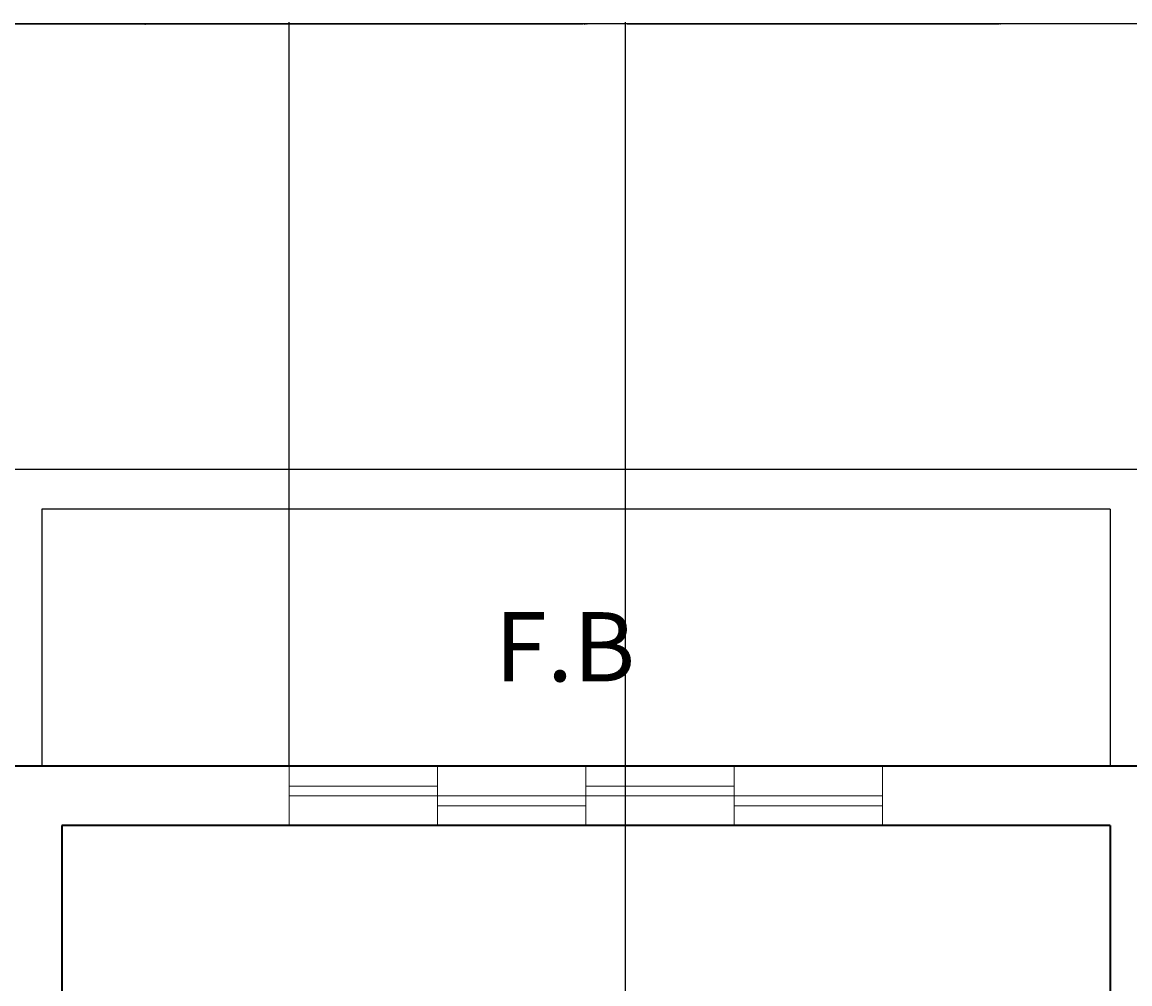
# Model space of a CAD drawing. Units: feet. Extents: x 105 to 1094, y -88 to 588.
# Tile 29 of 59: x 234 to 346, y 491 to 588. Entities that reach past the tile are written whole.
import ezdxf

# ---------------------------------------------------------------- set-up
doc = ezdxf.new("R2010")
doc.units = ezdxf.units.FT
doc.header["$MEASUREMENT"] = 0
for name, color, linetype, lineweight in [('A-ANNO-DIMS', 2, 'Continuous', 18), ('A-ANNO-TEXT', 7, 'Continuous', 18), ('A-FLOR-PROJ', 8, 'Continuous', 25), ('A-GLAZ', 4, 'Continuous', 18), ('A-WALL', 7, 'Continuous', 35)]:
    doc.layers.add(name, color=color, linetype=linetype, lineweight=lineweight)
doc.styles.get("Standard").update_dxf_attribs({"font": 'arial.ttf'})
doc.dimstyles.get("Standard").update_dxf_attribs({"dimtxt": 0.18, "dimasz": 0.18, "dimexe": 0.18, "dimexo": 0.0625, "dimgap": 0.09, "dimtad": 0, "dimtih": 1, "dimtoh": 1, "dimdec": 4, "dimzin": 0, "dimdsep": 46, "dimtxsty": 'Standard', "dimcen": 0.09, "dimadec": 0, "dimazin": 0, "dimtfac": 1, "dimtdec": 4, "dimtofl": 0, "dimtmove": 0, "dimatfit": 3, "dimfxl": 1, "dimtolj": 1, "dimtzin": 0, "dimarcsym": 0})

# ---------------------------------------------------------------- blocks, each defined once
blk = doc.blocks.new('WIN-FOUR-LIGHT')
for p, q in [((0, 0), (0, 6)), ((15, 0), (15, 6)), ((30, 0), (30, 6)), ((45, 0), (45, 6)), ((60, 0), (60, 6)), ((15, 4), (30, 4)), ((45, 4), (60, 4)), ((0, 3), (60, 3)), ((0, 2), (15, 2)), ((30, 2), (45, 2))]:
    blk.add_line(p, q)
blk = doc.blocks.new('*D21')
at = {"layer": 'A-ANNO-DIMS', "color": 0, "lineweight": -2, "transparency": 16777216}
for p, q in [((849.63, 543.08), (105.46, 543.08)), ((105.64, 542.9), (105.64, 250.26)), ((105.64, -42.74), (105.64, 249.9)), ((849.63, -42.92), (105.46, -42.92))]:
    blk.add_line(p, q, dxfattribs=at)
at = {"layer": 'A-ANNO-DIMS', "color": 0, "transparency": 16777216}
for points in [[(105.61, 542.9), (105.67, 542.9), (105.64, 543.08)], [(105.61, -42.74), (105.67, -42.74), (105.64, -42.92)]]:
    blk.add_solid(points, dxfattribs=at)
at = {"layer": 'Defpoints', "color": 0, "transparency": 16777216}
for p in [(105.64, 543.08), (849.69, 543.08), (849.69, -42.92)]:
    blk.add_point(p, dxfattribs=at)
at = {"layer": 'A-ANNO-DIMS', "color": 0, "transparency": 16777216, "insert": (105.64, 250.08), "char_height": 0.18, "attachment_point": 5}
blk.add_mtext('\\A1;586', dxfattribs=at)
blk = doc.blocks.new('*D23')
at = {"layer": 'A-ANNO-DIMS', "color": 0, "lineweight": -2, "transparency": 16777216}
for p, q in [((231.69, 543.14), (231.69, 588.31)), ((231.87, 588.13), (290.41, 588.13)), ((349.51, 588.13), (290.97, 588.13)), ((349.69, 543.14), (349.69, 588.31))]:
    blk.add_line(p, q, dxfattribs=at)
at = {"layer": 'A-ANNO-DIMS', "color": 0, "transparency": 16777216}
for points in [[(231.87, 588.16), (231.87, 588.1), (231.69, 588.13)], [(349.51, 588.16), (349.51, 588.1), (349.69, 588.13)]]:
    blk.add_solid(points, dxfattribs=at)
at = {"layer": 'Defpoints', "color": 0, "transparency": 16777216}
for p in [(349.69, 588.13), (231.69, 543.08), (349.69, 543.08)]:
    blk.add_point(p, dxfattribs=at)
at = {"layer": 'A-ANNO-DIMS', "color": 0, "transparency": 16777216, "insert": (290.69, 588.13), "char_height": 0.18, "attachment_point": 5}
blk.add_mtext('\\A1;118', dxfattribs=at)
blk = doc.blocks.new('*D38')
at = {"layer": 'A-ANNO-DIMS', "color": 0, "lineweight": -2, "transparency": 16777216}
for p, q in [((150.69, 224.14), (150.69, 588.31)), ((150.87, 588.13), (222.41, 588.13)), ((294.51, 588.13), (222.97, 588.13)), ((294.69, 224.14), (294.69, 588.31))]:
    blk.add_line(p, q, dxfattribs=at)
at = {"layer": 'A-ANNO-DIMS', "color": 0, "transparency": 16777216}
for points in [[(150.87, 588.16), (150.87, 588.1), (150.69, 588.13)], [(294.51, 588.16), (294.51, 588.1), (294.69, 588.13)]]:
    blk.add_solid(points, dxfattribs=at)
at = {"layer": 'Defpoints', "color": 0, "transparency": 16777216}
for p in [(294.69, 588.13), (150.69, 224.08), (294.69, 224.08)]:
    blk.add_point(p, dxfattribs=at)
at = {"layer": 'A-ANNO-DIMS', "color": 0, "transparency": 16777216, "insert": (222.69, 588.13), "char_height": 0.18, "attachment_point": 5}
blk.add_mtext('\\A1;144', dxfattribs=at)
blk = doc.blocks.new('*D39')
at = {"layer": 'A-ANNO-DIMS', "color": 0, "lineweight": -2, "transparency": 16777216}
for p, q in [((294.69, 204.14), (294.69, 588.31)), ((294.87, 588.13), (332.47, 588.13)), ((370.51, 588.13), (332.91, 588.13)), ((370.69, 204.14), (370.69, 588.31))]:
    blk.add_line(p, q, dxfattribs=at)
at = {"layer": 'A-ANNO-DIMS', "color": 0, "transparency": 16777216}
for points in [[(294.87, 588.16), (294.87, 588.1), (294.69, 588.13)], [(370.51, 588.16), (370.51, 588.1), (370.69, 588.13)]]:
    blk.add_solid(points, dxfattribs=at)
at = {"layer": 'Defpoints', "color": 0, "transparency": 16777216}
for p in [(370.69, 588.13), (294.69, 204.08), (370.69, 204.08)]:
    blk.add_point(p, dxfattribs=at)
at = {"layer": 'A-ANNO-DIMS', "color": 0, "transparency": 16777216, "insert": (332.69, 588.13), "char_height": 0.18, "attachment_point": 5}
blk.add_mtext('\\A1;76', dxfattribs=at)
blk = doc.blocks.new('*D42')
at = {"layer": 'A-ANNO-DIMS', "color": 0, "lineweight": -2, "transparency": 16777216}
for p, q in [((231.69, 513.14), (231.69, 588.31)), ((231.87, 588.13), (245.97, 588.13)), ((260.51, 588.13), (246.41, 588.13)), ((260.69, 513.14), (260.69, 588.31))]:
    blk.add_line(p, q, dxfattribs=at)
at = {"layer": 'A-ANNO-DIMS', "color": 0, "transparency": 16777216}
for points in [[(231.87, 588.16), (231.87, 588.1), (231.69, 588.13)], [(260.51, 588.16), (260.51, 588.1), (260.69, 588.13)]]:
    blk.add_solid(points, dxfattribs=at)
at = {"layer": 'Defpoints', "color": 0, "transparency": 16777216}
for p in [(260.69, 588.13), (231.69, 513.08), (260.69, 513.08)]:
    blk.add_point(p, dxfattribs=at)
at = {"layer": 'A-ANNO-DIMS', "color": 0, "transparency": 16777216, "insert": (246.19, 588.13), "char_height": 0.18, "attachment_point": 5}
blk.add_mtext('\\A1;29', dxfattribs=at)

msp = doc.modelspace()

# ---------------------------------------------------------------- linework, layer by layer
at = {"layer": 'A-FLOR-PROJ'}
for p, q in [((349.6883, 543.0812), (231.6883, 543.0812)), ((343.6883, 539.0812), (235.6883, 539.0812)), ((235.6883, 539.0812), (235.6883, 513.0812)), ((343.6883, 539.0812), (343.6883, 513.0812)), ((343.6883, 527.0812), (343.6883, 513.0812))]:
    msp.add_line(p, q, dxfattribs=at)
at = {"layer": 'A-WALL'}
for p, q in [((349.6883, 513.0812), (231.6883, 513.0812)), ((343.6883, 507.0812), (237.6883, 507.0812)), ((237.6883, 507.0812), (237.6883, 394.0812)), ((343.6883, 507.0812), (343.6883, 390.0812))]:
    msp.add_line(p, q, dxfattribs=at)

# ---------------------------------------------------------------- block references
at = {"layer": 'A-GLAZ', "extrusion": (0, 0, -1), "zscale": -1}
msp.add_blockref('WIN-FOUR-LIGHT', (-320.6886, 507.081), dxfattribs=at)

# ---------------------------------------------------------------- texts
at = {"layer": 'A-ANNO-TEXT', "insert": (337.7459, 528.6595), "char_height": 7, "attachment_point": 3}
msp.add_mtext_dynamic_manual_height_columns('\\pxqc;F.B ', width=98.34246, gutter_width=1, heights=[0], dxfattribs=at)

# ---------------------------------------------------------------- dimensions: what is measured, and where the dimension line sits
at = {"layer": 'A-ANNO-DIMS'}
for base, p1, p2, picture, middle in [((294.6883, 588.1312), (150.6883, 224.0812), (294.6883, 224.0812), '*D38', (222.6883, 588.1312)), ((349.6883, 588.1312), (231.6883, 543.0812), (349.6883, 543.0812), '*D23', (290.6883, 588.1312)), ((260.6883, 588.1312), (231.6883, 513.0812), (260.6883, 513.0812), '*D42', (246.1883, 588.1312)), ((370.6883, 588.1312), (294.6883, 204.0812), (370.6883, 204.0812), '*D39', (332.6883, 588.1312))]:
    dim = msp.add_linear_dim(base=base, p1=p1, p2=p2, dimstyle='Standard', override={"dimdec": 0, "dimlfac": 1, "dimrnd": 0, "dimzin": 0, "dimdsep": 46, "dimlunit": 2}, dxfattribs=at)
    dim.commit()
    dim.dimension.update_dxf_attribs({"geometry": picture, "text_midpoint": middle})
dim = msp.add_linear_dim(base=(105.6383, 543.0812), p1=(849.6883, -42.9188), p2=(849.6883, 543.0812), angle=90, dimstyle='Standard', override={"dimdec": 0, "dimlfac": 1, "dimrnd": 0, "dimzin": 0, "dimdsep": 46, "dimlunit": 2}, dxfattribs=at)
dim.commit()
dim.dimension.update_dxf_attribs({"geometry": '*D21', "text_midpoint": (105.6383, 250.0812)})

doc.saveas('drawing.dxf')
